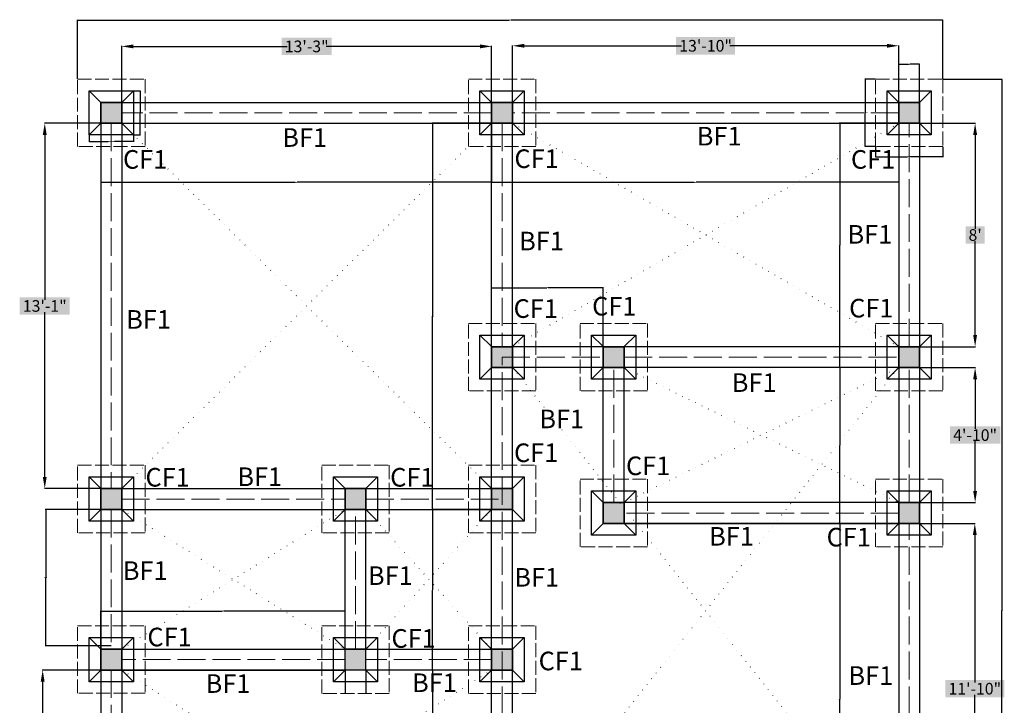
# Model space of a CAD drawing. Units: inches. Extents: x -35 to 832, y -515 to 219.
# Tile 7 of 7: x 409 to 832, y -75 to 219. Entities that reach past the tile are written whole.
import ezdxf

# ---------------------------------------------------------------- set-up
doc = ezdxf.new("R2010")
doc.units = ezdxf.units.IN
doc.header["$MEASUREMENT"] = 0
doc.linetypes.add('ACAD_ISO02W100', pattern=[15, 12, -3])
doc.linetypes.add('ACAD_ISO07W100', pattern=[3, 0, -3])
for name, color, linetype, lineweight in [('S-ANNO-DIMS', 2, 'Continuous', 18), ('S-ANNO-TEXT', 7, 'Continuous', 18), ('S-BEAM', 6, 'Continuous', 25), ('S-BEAM-CNTR', 2, 'ACAD_ISO02W100', 13), ('S-COLS', 4, 'Continuous', 35), ('S-COLS-PATT', 8, 'Continuous', 13), ('S-FNDN', 4, 'Continuous', 25), ('S-FNDN-HIDN', 7, 'ACAD_ISO02W100', 18), ('S-FNDN-REFR', 8, 'ACAD_ISO07W100', 13)]:
    doc.layers.add(name, color=color, linetype=linetype, lineweight=lineweight)
doc.styles.get("Standard").update_dxf_attribs({"font": 'arial.ttf'})
doc.dimstyles.get("Standard").update_dxf_attribs({"dimtxt": 0.18, "dimasz": 0.18, "dimexe": 0.18, "dimexo": 0.0625, "dimgap": 0.09, "dimtad": 0, "dimtih": 1, "dimtoh": 1, "dimdec": 1, "dimzin": 0, "dimdsep": 46, "dimlunit": 4, "dimtxsty": 'Standard', "dimcen": 0.09, "dimclrd": 211, "dimclre": 4, "dimclrt": 3, "dimadec": 0, "dimazin": 0, "dimtfac": 0.5, "dimtdec": 1, "dimtofl": 0, "dimtmove": 0, "dimatfit": 3, "dimfxl": 1, "dimtfill": 2, "dimtfillclr": 61, "dimtolj": 1, "dimtzin": 0, "dimarcsym": 0})

# ---------------------------------------------------------------- blocks, each defined once
blk = doc.blocks.new('*D31')
at = {"layer": 'Defpoints', "color": 0, "transparency": 16777216}
for p in [(786.57, 2.92), (819.29, 2.92), (786.57, -139.08)]:
    blk.add_point(p, dxfattribs=at)
at = {"layer": 'S-ANNO-DIMS', "color": 0, "lineweight": -2, "transparency": 16777216}
for p, q in [((786.63, 2.92), (819.47, 2.92)), ((819.29, -2.08), (819.29, -65.43)), ((819.29, -134.08), (819.29, -70.72)), ((786.63, -139.08), (819.47, -139.08))]:
    blk.add_line(p, q, dxfattribs=at)
at = {"layer": 'S-ANNO-DIMS', "color": 0, "transparency": 16777216}
for points in [[(818.46, -2.08), (820.13, -2.08), (819.29, 2.92)], [(818.46, -134.08), (820.13, -134.08), (819.29, -139.08)]]:
    blk.add_solid(points, dxfattribs=at)
at = {"layer": 'S-ANNO-DIMS', "color": 0, "transparency": 16777216, "insert": (819.29, -68.08), "char_height": 5, "attachment_point": 5, "bg_fill": 1, "box_fill_scale": 1.25, "bg_fill_color": 61, "bg_fill_transparency": 0}
blk.add_mtext('\\A1;11\'-10"', dxfattribs=at)
blk = doc.blocks.new('*D32')
at = {"layer": 'Defpoints', "color": 0, "transparency": 16777216}
for p in [(791.07, 69.92), (819.43, 69.92), (791.07, 11.92)]:
    blk.add_point(p, dxfattribs=at)
at = {"layer": 'S-ANNO-DIMS', "color": 0, "lineweight": -2, "transparency": 16777216}
for p, q in [((791.13, 69.92), (819.61, 69.92)), ((819.43, 64.92), (819.43, 43.57)), ((819.43, 16.92), (819.43, 38.28)), ((791.13, 11.92), (819.61, 11.92))]:
    blk.add_line(p, q, dxfattribs=at)
at = {"layer": 'S-ANNO-DIMS', "color": 0, "transparency": 16777216}
for points in [[(818.6, 64.92), (820.26, 64.92), (819.43, 69.92)], [(818.6, 16.92), (820.26, 16.92), (819.43, 11.92)]]:
    blk.add_solid(points, dxfattribs=at)
at = {"layer": 'S-ANNO-DIMS', "color": 0, "transparency": 16777216, "insert": (819.43, 40.92), "char_height": 5, "attachment_point": 5, "bg_fill": 1, "box_fill_scale": 1.25, "bg_fill_color": 61, "bg_fill_transparency": 0}
blk.add_mtext('\\A1;4\'-10"', dxfattribs=at)
blk = doc.blocks.new('*D33')
at = {"layer": 'Defpoints', "color": 0, "transparency": 16777216}
for p in [(791.07, 174.92), (819.43, 174.92), (791.07, 78.92)]:
    blk.add_point(p, dxfattribs=at)
at = {"layer": 'S-ANNO-DIMS', "color": 0, "lineweight": -2, "transparency": 16777216}
for p, q in [((791.13, 174.92), (819.61, 174.92)), ((819.43, 169.92), (819.43, 129.57)), ((819.43, 83.92), (819.43, 124.28)), ((791.13, 78.92), (819.61, 78.92))]:
    blk.add_line(p, q, dxfattribs=at)
at = {"layer": 'S-ANNO-DIMS', "color": 0, "transparency": 16777216}
for points in [[(818.6, 169.92), (820.27, 169.92), (819.43, 174.92)], [(818.6, 83.92), (820.27, 83.92), (819.43, 78.92)]]:
    blk.add_solid(points, dxfattribs=at)
at = {"layer": 'S-ANNO-DIMS', "color": 0, "transparency": 16777216, "insert": (819.43, 126.92), "char_height": 5, "attachment_point": 5, "bg_fill": 1, "box_fill_scale": 1.25, "bg_fill_color": 61, "bg_fill_transparency": 0}
blk.add_mtext("\\A1;8'", dxfattribs=at)
blk = doc.blocks.new('*D34')
at = {"layer": 'Defpoints', "color": 0, "transparency": 16777216}
for p in [(611.57, 207.98), (452.57, 179.42), (611.57, 179.42)]:
    blk.add_point(p, dxfattribs=at)
at = {"layer": 'S-ANNO-DIMS', "color": 0, "lineweight": -2, "transparency": 16777216}
for p, q in [((452.57, 179.49), (452.57, 208.16)), ((457.57, 207.98), (523.63, 207.98)), ((606.57, 207.98), (540.51, 207.98)), ((611.57, 179.49), (611.57, 208.16))]:
    blk.add_line(p, q, dxfattribs=at)
at = {"layer": 'S-ANNO-DIMS', "color": 0, "transparency": 16777216}
for points in [[(457.57, 208.81), (457.57, 207.14), (452.57, 207.98)], [(606.57, 208.81), (606.57, 207.14), (611.57, 207.98)]]:
    blk.add_solid(points, dxfattribs=at)
at = {"layer": 'S-ANNO-DIMS', "color": 0, "transparency": 16777216, "insert": (532.07, 207.98), "char_height": 5, "attachment_point": 5, "bg_fill": 1, "box_fill_scale": 1.25, "bg_fill_color": 61, "bg_fill_transparency": 0}
blk.add_mtext('\\A1;13\'-3"', dxfattribs=at)
blk = doc.blocks.new('*D35')
at = {"layer": 'Defpoints', "color": 0, "transparency": 16777216}
for p in [(786.57, 208.24), (620.57, 179.42), (786.57, 179.42)]:
    blk.add_point(p, dxfattribs=at)
at = {"layer": 'S-ANNO-DIMS', "color": 0, "lineweight": -2, "transparency": 16777216}
for p, q in [((620.57, 179.49), (620.57, 208.42)), ((625.57, 208.24), (693.19, 208.24)), ((781.57, 208.24), (713.96, 208.24)), ((786.57, 179.49), (786.57, 208.42))]:
    blk.add_line(p, q, dxfattribs=at)
at = {"layer": 'S-ANNO-DIMS', "color": 0, "transparency": 16777216}
for points in [[(625.57, 209.07), (625.57, 207.41), (620.57, 208.24)], [(781.57, 209.07), (781.57, 207.41), (786.57, 208.24)]]:
    blk.add_solid(points, dxfattribs=at)
at = {"layer": 'S-ANNO-DIMS', "color": 0, "transparency": 16777216, "insert": (703.57, 208.24), "char_height": 5, "attachment_point": 5, "bg_fill": 1, "box_fill_scale": 1.25, "bg_fill_color": 61, "bg_fill_transparency": 0}
blk.add_mtext('\\A1;13\'-10"', dxfattribs=at)
blk = doc.blocks.new('*D36')
at = {"layer": 'Defpoints', "color": 0, "transparency": 16777216}
for p in [(448.07, 174.92), (419.47, 17.92), (448.07, 17.92)]:
    blk.add_point(p, dxfattribs=at)
at = {"layer": 'S-ANNO-DIMS', "color": 0, "lineweight": -2, "transparency": 16777216}
for p, q in [((448.01, 174.92), (419.29, 174.92)), ((419.47, 169.92), (419.47, 99.07)), ((419.47, 22.92), (419.47, 93.78)), ((448.01, 17.92), (419.29, 17.92))]:
    blk.add_line(p, q, dxfattribs=at)
at = {"layer": 'S-ANNO-DIMS', "color": 0, "transparency": 16777216}
for points in [[(418.63, 169.92), (420.3, 169.92), (419.47, 174.92)], [(418.63, 22.92), (420.3, 22.92), (419.47, 17.92)]]:
    blk.add_solid(points, dxfattribs=at)
at = {"layer": 'S-ANNO-DIMS', "color": 0, "transparency": 16777216, "insert": (419.47, 96.42), "char_height": 5, "attachment_point": 5, "bg_fill": 1, "box_fill_scale": 1.25, "bg_fill_color": 61, "bg_fill_transparency": 0}
blk.add_mtext('\\A1;13\'-1"', dxfattribs=at)
blk = doc.blocks.new('*D37')
at = {"layer": 'Defpoints', "color": 0, "transparency": 16777216}
for p in [(448.07, 8.92), (419.88, -49.73), (448.07, -49.73)]:
    blk.add_point(p, dxfattribs=at)
at = {"layer": 'S-ANNO-DIMS', "color": 0, "lineweight": -2, "transparency": 16777216}
for p, q in [((448.01, 8.92), (419.7, 8.92)), ((419.88, 8.74), (419.88, -20.21)), ((419.88, -49.55), (419.88, -20.6)), ((448.01, -49.73), (419.7, -49.73))]:
    blk.add_line(p, q, dxfattribs=at)
at = {"layer": 'S-ANNO-DIMS', "color": 0, "transparency": 16777216}
for points in [[(419.85, 8.74), (419.91, 8.74), (419.88, 8.92)], [(419.85, -49.55), (419.91, -49.55), (419.88, -49.73)]]:
    blk.add_solid(points, dxfattribs=at)
at = {"layer": 'S-ANNO-DIMS', "color": 0, "transparency": 16777216, "insert": (419.88, -20.4), "char_height": 0.18, "attachment_point": 5, "bg_fill": 1, "box_fill_scale": 1.25, "bg_fill_color": 61, "bg_fill_transparency": 0}
blk.add_mtext('\\A1;4\'-10{\\H0.5x;\\S1/2;}"', dxfattribs=at)
blk = doc.blocks.new('*D38')
at = {"layer": 'Defpoints', "color": 0, "transparency": 16777216}
for p in [(448.07, -60.08), (418.57, -161.08), (448.07, -161.08)]:
    blk.add_point(p, dxfattribs=at)
at = {"layer": 'S-ANNO-DIMS', "color": 0, "lineweight": -2, "transparency": 16777216}
for p, q in [((448.01, -60.08), (418.39, -60.08)), ((418.57, -65.08), (418.57, -107.93)), ((418.57, -156.08), (418.57, -113.22)), ((448.01, -161.08), (418.39, -161.08))]:
    blk.add_line(p, q, dxfattribs=at)
at = {"layer": 'S-ANNO-DIMS', "color": 0, "transparency": 16777216}
for points in [[(417.74, -65.08), (419.41, -65.08), (418.57, -60.08)], [(417.74, -156.08), (419.41, -156.08), (418.57, -161.08)]]:
    blk.add_solid(points, dxfattribs=at)
at = {"layer": 'S-ANNO-DIMS', "color": 0, "transparency": 16777216, "insert": (418.57, -110.58), "char_height": 5, "attachment_point": 5, "bg_fill": 1, "box_fill_scale": 1.25, "bg_fill_color": 61, "bg_fill_transparency": 0}
blk.add_mtext('\\A1;8\'-5"', dxfattribs=at)
blk = doc.blocks.new('CF1-TAPERED-FOOTING')
for p, q in [((0, 19), (19, 19)), ((0, 0), (0, 19)), ((0, 19), (5, 14)), ((14, 14), (19, 19)), ((19, 19), (19, 0)), ((0, 0), (5, 5)), ((14, 5), (19, 0)), ((19, 0), (0, 0))]:
    blk.add_line(p, q)
blk = doc.blocks.new('CF1-FOOTING-LIMIT')
at = {"ltscale": 0.5}
for p, q in [((0, 29), (29, 29)), ((0, 0), (0, 29)), ((29, 29), (29, 0)), ((29, 0), (0, 0))]:
    blk.add_line(p, q, dxfattribs=at)
blk = doc.blocks.new('*D57')
at = {"layer": 'Defpoints', "color": 0, "transparency": 16777216}
for p in [(438.57, 169.92), (457.57, 169.92), (457.57, 167.07)]:
    blk.add_point(p, dxfattribs=at)
at = {"layer": 'S-ANNO-DIMS', "color": 4, "lineweight": -2, "transparency": 16777216}
for p, q in [((438.57, 169.86), (438.57, 166.89)), ((457.57, 169.86), (457.57, 166.89))]:
    blk.add_line(p, q, dxfattribs=at)
at = {"layer": 'S-ANNO-DIMS', "color": 211, "lineweight": -2, "transparency": 16777216}
for p, q in [((438.75, 167.07), (446.71, 167.07)), ((457.39, 167.07), (449.44, 167.07))]:
    blk.add_line(p, q, dxfattribs=at)
at = {"layer": 'S-ANNO-DIMS', "color": 211, "transparency": 16777216}
for points in [[(438.75, 167.1), (438.75, 167.04), (438.57, 167.07)], [(457.39, 167.1), (457.39, 167.04), (457.57, 167.07)]]:
    blk.add_solid(points, dxfattribs=at)
at = {"layer": 'S-ANNO-DIMS', "color": 3, "transparency": 16777216, "insert": (448.07, 167.07), "char_height": 0.18, "attachment_point": 5, "bg_fill": 1, "box_fill_scale": 1.25, "bg_fill_color": 61, "bg_fill_transparency": 0}
blk.add_mtext('\\A1;CF1 TAPER 1\'-7" TYP.', dxfattribs=at)
blk = doc.blocks.new('*D58')
at = {"layer": 'Defpoints', "color": 0, "transparency": 16777216}
for p in [(457.57, 188.92), (460.42, 188.92), (457.57, 169.92)]:
    blk.add_point(p, dxfattribs=at)
at = {"layer": 'S-ANNO-DIMS', "color": 4, "lineweight": -2, "transparency": 16777216}
for p, q in [((457.63, 188.92), (460.6, 188.92)), ((457.63, 169.92), (460.6, 169.92))]:
    blk.add_line(p, q, dxfattribs=at)
at = {"layer": 'S-ANNO-DIMS', "color": 211, "lineweight": -2, "transparency": 16777216}
for p, q in [((460.42, 188.74), (460.42, 179.61)), ((460.42, 170.1), (460.42, 179.24))]:
    blk.add_line(p, q, dxfattribs=at)
at = {"layer": 'S-ANNO-DIMS', "color": 211, "transparency": 16777216}
for points in [[(460.39, 188.74), (460.45, 188.74), (460.42, 188.92)], [(460.39, 170.1), (460.45, 170.1), (460.42, 169.92)]]:
    blk.add_solid(points, dxfattribs=at)
at = {"layer": 'S-ANNO-DIMS', "color": 3, "transparency": 16777216, "insert": (460.42, 179.42), "char_height": 0.18, "attachment_point": 5, "bg_fill": 1, "box_fill_scale": 1.25, "bg_fill_color": 61, "bg_fill_transparency": 0}
blk.add_mtext('\\A1;1\'-7" TYP.', dxfattribs=at)
blk = doc.blocks.new('*D59')
at = {"layer": 'Defpoints', "color": 0, "transparency": 16777216}
for p in [(772.22, 193.92), (776.57, 193.92), (776.57, 164.92)]:
    blk.add_point(p, dxfattribs=at)
at = {"layer": 'S-ANNO-DIMS', "color": 4, "lineweight": -2, "transparency": 16777216}
for p, q in [((776.51, 193.92), (772.04, 193.92)), ((776.51, 164.92), (772.04, 164.92))]:
    blk.add_line(p, q, dxfattribs=at)
at = {"layer": 'S-ANNO-DIMS', "color": 211, "lineweight": -2, "transparency": 16777216}
for p, q in [((772.22, 193.74), (772.22, 179.61)), ((772.22, 165.1), (772.22, 179.24))]:
    blk.add_line(p, q, dxfattribs=at)
at = {"layer": 'S-ANNO-DIMS', "color": 211, "transparency": 16777216}
for points in [[(772.19, 193.74), (772.25, 193.74), (772.22, 193.92)], [(772.19, 165.1), (772.25, 165.1), (772.22, 164.92)]]:
    blk.add_solid(points, dxfattribs=at)
at = {"layer": 'S-ANNO-DIMS', "color": 3, "transparency": 16777216, "insert": (772.22, 179.42), "char_height": 0.18, "attachment_point": 5, "bg_fill": 1, "box_fill_scale": 1.25, "bg_fill_color": 61, "bg_fill_transparency": 0}
blk.add_mtext('\\A1;CF1 LIMIT 2\'-5" TYP.', dxfattribs=at)
blk = doc.blocks.new('*D60')
at = {"layer": 'Defpoints', "color": 0, "transparency": 16777216}
for p in [(776.57, 164.92), (805.57, 164.92), (776.57, 160.57)]:
    blk.add_point(p, dxfattribs=at)
at = {"layer": 'S-ANNO-DIMS', "color": 4, "lineweight": -2, "transparency": 16777216}
for p, q in [((776.57, 164.86), (776.57, 160.39)), ((805.57, 164.86), (805.57, 160.39))]:
    blk.add_line(p, q, dxfattribs=at)
at = {"layer": 'S-ANNO-DIMS', "color": 211, "lineweight": -2, "transparency": 16777216}
for p, q in [((776.75, 160.57), (790.43, 160.57)), ((805.39, 160.57), (791.71, 160.57))]:
    blk.add_line(p, q, dxfattribs=at)
at = {"layer": 'S-ANNO-DIMS', "color": 211, "transparency": 16777216}
for points in [[(776.75, 160.6), (776.75, 160.54), (776.57, 160.57)], [(805.39, 160.6), (805.39, 160.54), (805.57, 160.57)]]:
    blk.add_solid(points, dxfattribs=at)
at = {"layer": 'S-ANNO-DIMS', "color": 3, "transparency": 16777216, "insert": (791.07, 160.57), "char_height": 0.18, "attachment_point": 5, "bg_fill": 1, "box_fill_scale": 1.25, "bg_fill_color": 61, "bg_fill_transparency": 0}
blk.add_mtext('\\A1;2\'-5" TYP.', dxfattribs=at)
blk = doc.blocks.new('*D136')
at = {"layer": 'Defpoints', "color": 0, "transparency": 16777216}
for p in [(548.57, -34.73), (443.57, -60.08), (548.57, -60.08)]:
    blk.add_point(p, dxfattribs=at)
at = {"layer": 'S-ANNO-DIMS', "color": 4, "lineweight": -2, "transparency": 16777216}
for p, q in [((443.57, -60.01), (443.57, -34.55)), ((548.57, -60.01), (548.57, -34.55))]:
    blk.add_line(p, q, dxfattribs=at)
at = {"layer": 'S-ANNO-DIMS', "color": 211, "lineweight": -2, "transparency": 16777216}
for p, q in [((443.75, -34.73), (495.74, -34.73)), ((548.39, -34.73), (496.4, -34.73))]:
    blk.add_line(p, q, dxfattribs=at)
at = {"layer": 'S-ANNO-DIMS', "color": 211, "transparency": 16777216}
for points in [[(443.75, -34.7), (443.75, -34.76), (443.57, -34.73)], [(548.39, -34.7), (548.39, -34.76), (548.57, -34.73)]]:
    blk.add_solid(points, dxfattribs=at)
at = {"layer": 'S-ANNO-DIMS', "color": 3, "transparency": 16777216, "insert": (496.07, -34.73), "char_height": 0.18, "attachment_point": 5, "bg_fill": 1, "box_fill_scale": 1.25, "bg_fill_color": 61, "bg_fill_transparency": 0}
blk.add_mtext('\\A1;8\'-9"', dxfattribs=at)
blk = doc.blocks.new('*D137')
at = {"layer": 'Defpoints', "color": 0, "transparency": 16777216}
for p in [(659.57, 104.27), (611.57, 78.92), (659.57, 78.92)]:
    blk.add_point(p, dxfattribs=at)
at = {"layer": 'S-ANNO-DIMS', "color": 4, "lineweight": -2, "transparency": 16777216}
for p, q in [((611.57, 78.99), (611.57, 104.45)), ((659.57, 78.99), (659.57, 104.45))]:
    blk.add_line(p, q, dxfattribs=at)
at = {"layer": 'S-ANNO-DIMS', "color": 211, "lineweight": -2, "transparency": 16777216}
for p, q in [((611.75, 104.27), (635.24, 104.27)), ((659.39, 104.27), (635.9, 104.27))]:
    blk.add_line(p, q, dxfattribs=at)
at = {"layer": 'S-ANNO-DIMS', "color": 211, "transparency": 16777216}
for points in [[(611.75, 104.3), (611.75, 104.24), (611.57, 104.27)], [(659.39, 104.3), (659.39, 104.24), (659.57, 104.27)]]:
    blk.add_solid(points, dxfattribs=at)
at = {"layer": 'S-ANNO-DIMS', "color": 3, "transparency": 16777216, "insert": (635.57, 104.27), "char_height": 0.18, "attachment_point": 5, "bg_fill": 1, "box_fill_scale": 1.25, "bg_fill_color": 61, "bg_fill_transparency": 0}
blk.add_mtext('\\A1;4\'-0"', dxfattribs=at)
blk = doc.blocks.new('*D138')
at = {"layer": 'Defpoints', "color": 0, "transparency": 16777216}
for p in [(795.57, 200.27), (786.57, 174.92), (795.57, 174.92)]:
    blk.add_point(p, dxfattribs=at)
at = {"layer": 'S-ANNO-DIMS', "color": 4, "lineweight": -2, "transparency": 16777216}
for p, q in [((786.57, 174.99), (786.57, 200.45)), ((795.57, 174.99), (795.57, 200.45))]:
    blk.add_line(p, q, dxfattribs=at)
at = {"layer": 'S-ANNO-DIMS', "color": 211, "lineweight": -2, "transparency": 16777216}
for p, q in [((786.75, 200.27), (790.74, 200.27)), ((795.39, 200.27), (791.4, 200.27))]:
    blk.add_line(p, q, dxfattribs=at)
at = {"layer": 'S-ANNO-DIMS', "color": 211, "transparency": 16777216}
for points in [[(786.75, 200.3), (786.75, 200.24), (786.57, 200.27)], [(795.39, 200.3), (795.39, 200.24), (795.57, 200.27)]]:
    blk.add_solid(points, dxfattribs=at)
at = {"layer": 'S-ANNO-DIMS', "color": 3, "transparency": 16777216, "insert": (791.07, 200.27), "char_height": 0.18, "attachment_point": 5, "bg_fill": 1, "box_fill_scale": 1.25, "bg_fill_color": 61, "bg_fill_transparency": 0}
blk.add_mtext('\\A1;0\'-9"', dxfattribs=at)
blk = doc.blocks.new('*D139')
at = {"layer": 'Defpoints', "color": 0, "transparency": 16777216}
for p in [(805.57, 219.27), (433.57, 193.92), (805.57, 193.92)]:
    blk.add_point(p, dxfattribs=at)
at = {"layer": 'S-ANNO-DIMS', "color": 4, "lineweight": -2, "transparency": 16777216}
for p, q in [((433.57, 193.99), (433.57, 219.45)), ((805.57, 193.99), (805.57, 219.45))]:
    blk.add_line(p, q, dxfattribs=at)
at = {"layer": 'S-ANNO-DIMS', "color": 211, "lineweight": -2, "transparency": 16777216}
for p, q in [((433.75, 219.27), (619.17, 219.27)), ((805.39, 219.27), (619.97, 219.27))]:
    blk.add_line(p, q, dxfattribs=at)
at = {"layer": 'S-ANNO-DIMS', "color": 211, "transparency": 16777216}
for points in [[(433.75, 219.3), (433.75, 219.24), (433.57, 219.27)], [(805.39, 219.3), (805.39, 219.24), (805.57, 219.27)]]:
    blk.add_solid(points, dxfattribs=at)
at = {"layer": 'S-ANNO-DIMS', "color": 3, "transparency": 16777216, "insert": (619.57, 219.27), "char_height": 0.18, "attachment_point": 5, "bg_fill": 1, "box_fill_scale": 1.25, "bg_fill_color": 61, "bg_fill_transparency": 0}
blk.add_mtext('\\A1;31\'-0"', dxfattribs=at)
blk = doc.blocks.new('*D140')
at = {"layer": 'Defpoints', "color": 0, "transparency": 16777216}
for p in [(805.57, 193.92), (805.57, -263.08), (830.92, -263.08)]:
    blk.add_point(p, dxfattribs=at)
at = {"layer": 'S-ANNO-DIMS', "color": 4, "lineweight": -2, "transparency": 16777216}
for p, q in [((805.63, 193.92), (831.1, 193.92)), ((805.63, -263.08), (831.1, -263.08))]:
    blk.add_line(p, q, dxfattribs=at)
at = {"layer": 'S-ANNO-DIMS', "color": 211, "lineweight": -2, "transparency": 16777216}
for p, q in [((830.92, 193.74), (830.92, -34.39)), ((830.92, -262.9), (830.92, -34.76))]:
    blk.add_line(p, q, dxfattribs=at)
at = {"layer": 'S-ANNO-DIMS', "color": 211, "transparency": 16777216}
for points in [[(830.89, 193.74), (830.95, 193.74), (830.92, 193.92)], [(830.89, -262.9), (830.95, -262.9), (830.92, -263.08)]]:
    blk.add_solid(points, dxfattribs=at)
at = {"layer": 'S-ANNO-DIMS', "color": 3, "transparency": 16777216, "insert": (830.92, -34.58), "char_height": 0.18, "attachment_point": 5, "bg_fill": 1, "box_fill_scale": 1.25, "bg_fill_color": 61, "bg_fill_transparency": 0}
blk.add_mtext('\\A1;38\'-1"', dxfattribs=at)
blk = doc.blocks.new('*D141')
at = {"layer": 'Defpoints', "color": 0, "transparency": 16777216}
for p in [(443.57, 174.92), (611.57, 174.92), (443.57, 149.57)]:
    blk.add_point(p, dxfattribs=at)
at = {"layer": 'S-ANNO-DIMS', "color": 4, "lineweight": -2, "transparency": 16777216}
for p, q in [((443.57, 174.86), (443.57, 149.39)), ((611.57, 174.86), (611.57, 149.39))]:
    blk.add_line(p, q, dxfattribs=at)
at = {"layer": 'S-ANNO-DIMS', "color": 211, "lineweight": -2, "transparency": 16777216}
for p, q in [((443.75, 149.57), (527.18, 149.57)), ((611.39, 149.57), (527.96, 149.57))]:
    blk.add_line(p, q, dxfattribs=at)
at = {"layer": 'S-ANNO-DIMS', "color": 211, "transparency": 16777216}
for points in [[(443.75, 149.6), (443.75, 149.54), (443.57, 149.57)], [(611.39, 149.6), (611.39, 149.54), (611.57, 149.57)]]:
    blk.add_solid(points, dxfattribs=at)
at = {"layer": 'S-ANNO-DIMS', "color": 3, "transparency": 16777216, "insert": (527.57, 149.57), "char_height": 0.18, "attachment_point": 5, "bg_fill": 1, "box_fill_scale": 1.25, "bg_fill_color": 61, "bg_fill_transparency": 0}
blk.add_mtext('\\A1;14\'-0"', dxfattribs=at)
blk = doc.blocks.new('*D142')
at = {"layer": 'Defpoints', "color": 0, "transparency": 16777216}
for p in [(611.57, 174.92), (786.57, 174.92), (611.57, 149.57)]:
    blk.add_point(p, dxfattribs=at)
at = {"layer": 'S-ANNO-DIMS', "color": 4, "lineweight": -2, "transparency": 16777216}
for p, q in [((611.57, 174.86), (611.57, 149.39)), ((786.57, 174.86), (786.57, 149.39))]:
    blk.add_line(p, q, dxfattribs=at)
at = {"layer": 'S-ANNO-DIMS', "color": 211, "lineweight": -2, "transparency": 16777216}
for p, q in [((611.75, 149.57), (698.68, 149.57)), ((786.39, 149.57), (699.46, 149.57))]:
    blk.add_line(p, q, dxfattribs=at)
at = {"layer": 'S-ANNO-DIMS', "color": 211, "transparency": 16777216}
for points in [[(611.75, 149.6), (611.75, 149.54), (611.57, 149.57)], [(786.39, 149.6), (786.39, 149.54), (786.57, 149.57)]]:
    blk.add_solid(points, dxfattribs=at)
at = {"layer": 'S-ANNO-DIMS', "color": 3, "transparency": 16777216, "insert": (699.07, 149.57), "char_height": 0.18, "attachment_point": 5, "bg_fill": 1, "box_fill_scale": 1.25, "bg_fill_color": 61, "bg_fill_transparency": 0}
blk.add_mtext('\\A1;14\'-7"', dxfattribs=at)
blk = doc.blocks.new('*D143')
at = {"layer": 'Defpoints', "color": 0, "transparency": 16777216}
for p in [(586.22, 174.92), (611.57, 174.92), (611.57, 8.92)]:
    blk.add_point(p, dxfattribs=at)
at = {"layer": 'S-ANNO-DIMS', "color": 4, "lineweight": -2, "transparency": 16777216}
for p, q in [((611.51, 174.92), (586.04, 174.92)), ((611.51, 8.92), (586.04, 8.92))]:
    blk.add_line(p, q, dxfattribs=at)
at = {"layer": 'S-ANNO-DIMS', "color": 211, "lineweight": -2, "transparency": 16777216}
for p, q in [((586.22, 174.74), (586.22, 92.11)), ((586.22, 9.1), (586.22, 91.74))]:
    blk.add_line(p, q, dxfattribs=at)
at = {"layer": 'S-ANNO-DIMS', "color": 211, "transparency": 16777216}
for points in [[(586.19, 174.74), (586.25, 174.74), (586.22, 174.92)], [(586.19, 9.1), (586.25, 9.1), (586.22, 8.92)]]:
    blk.add_solid(points, dxfattribs=at)
at = {"layer": 'S-ANNO-DIMS', "color": 3, "transparency": 16777216, "insert": (586.22, 91.92), "char_height": 0.18, "attachment_point": 5, "bg_fill": 1, "box_fill_scale": 1.25, "bg_fill_color": 61, "bg_fill_transparency": 0}
blk.add_mtext('\\A1;13\'-10"', dxfattribs=at)
blk = doc.blocks.new('*D144')
at = {"layer": 'Defpoints', "color": 0, "transparency": 16777216}
for p in [(586.22, 8.92), (611.57, 8.92), (611.57, -60.08)]:
    blk.add_point(p, dxfattribs=at)
at = {"layer": 'S-ANNO-DIMS', "color": 4, "lineweight": -2, "transparency": 16777216}
for p, q in [((611.51, 8.92), (586.04, 8.92)), ((611.51, -60.08), (586.04, -60.08))]:
    blk.add_line(p, q, dxfattribs=at)
at = {"layer": 'S-ANNO-DIMS', "color": 211, "lineweight": -2, "transparency": 16777216}
for p, q in [((586.22, 8.74), (586.22, -25.39)), ((586.22, -59.9), (586.22, -25.76))]:
    blk.add_line(p, q, dxfattribs=at)
at = {"layer": 'S-ANNO-DIMS', "color": 211, "transparency": 16777216}
for points in [[(586.19, 8.74), (586.25, 8.74), (586.22, 8.92)], [(586.19, -59.9), (586.25, -59.9), (586.22, -60.08)]]:
    blk.add_solid(points, dxfattribs=at)
at = {"layer": 'S-ANNO-DIMS', "color": 3, "transparency": 16777216, "insert": (586.22, -25.58), "char_height": 0.18, "attachment_point": 5, "bg_fill": 1, "box_fill_scale": 1.25, "bg_fill_color": 61, "bg_fill_transparency": 0}
blk.add_mtext('\\A1;5\'-9"', dxfattribs=at)
blk = doc.blocks.new('*D145')
at = {"layer": 'Defpoints', "color": 0, "transparency": 16777216}
for p in [(586.22, -60.08), (611.57, -60.08), (611.57, -170.08)]:
    blk.add_point(p, dxfattribs=at)
at = {"layer": 'S-ANNO-DIMS', "color": 4, "lineweight": -2, "transparency": 16777216}
for p, q in [((611.51, -60.08), (586.04, -60.08)), ((611.51, -170.08), (586.04, -170.08))]:
    blk.add_line(p, q, dxfattribs=at)
at = {"layer": 'S-ANNO-DIMS', "color": 211, "lineweight": -2, "transparency": 16777216}
for p, q in [((586.22, -60.26), (586.22, -114.89)), ((586.22, -169.9), (586.22, -115.26))]:
    blk.add_line(p, q, dxfattribs=at)
at = {"layer": 'S-ANNO-DIMS', "color": 211, "transparency": 16777216}
for points in [[(586.19, -60.26), (586.25, -60.26), (586.22, -60.08)], [(586.19, -169.9), (586.25, -169.9), (586.22, -170.08)]]:
    blk.add_solid(points, dxfattribs=at)
at = {"layer": 'S-ANNO-DIMS', "color": 3, "transparency": 16777216, "insert": (586.22, -115.08), "char_height": 0.18, "attachment_point": 5, "bg_fill": 1, "box_fill_scale": 1.25, "bg_fill_color": 61, "bg_fill_transparency": 0}
blk.add_mtext('\\A1;9\'-2"', dxfattribs=at)
blk = doc.blocks.new('*D146')
at = {"layer": 'Defpoints', "color": 0, "transparency": 16777216}
for p in [(761.22, 174.92), (786.57, 174.92), (786.57, 69.92)]:
    blk.add_point(p, dxfattribs=at)
at = {"layer": 'S-ANNO-DIMS', "color": 4, "lineweight": -2, "transparency": 16777216}
for p, q in [((786.51, 174.92), (761.04, 174.92)), ((786.51, 69.92), (761.04, 69.92))]:
    blk.add_line(p, q, dxfattribs=at)
at = {"layer": 'S-ANNO-DIMS', "color": 211, "lineweight": -2, "transparency": 16777216}
for p, q in [((761.22, 174.74), (761.22, 122.61)), ((761.22, 70.1), (761.22, 122.24))]:
    blk.add_line(p, q, dxfattribs=at)
at = {"layer": 'S-ANNO-DIMS', "color": 211, "transparency": 16777216}
for points in [[(761.19, 174.74), (761.25, 174.74), (761.22, 174.92)], [(761.19, 70.1), (761.25, 70.1), (761.22, 69.92)]]:
    blk.add_solid(points, dxfattribs=at)
at = {"layer": 'S-ANNO-DIMS', "color": 3, "transparency": 16777216, "insert": (761.22, 122.42), "char_height": 0.18, "attachment_point": 5, "bg_fill": 1, "box_fill_scale": 1.25, "bg_fill_color": 61, "bg_fill_transparency": 0}
blk.add_mtext('\\A1;8\'-9"', dxfattribs=at)
blk = doc.blocks.new('*D147')
at = {"layer": 'Defpoints', "color": 0, "transparency": 16777216}
for p in [(761.22, 69.92), (786.57, 69.92), (786.57, 2.92)]:
    blk.add_point(p, dxfattribs=at)
at = {"layer": 'S-ANNO-DIMS', "color": 4, "lineweight": -2, "transparency": 16777216}
for p, q in [((786.51, 69.92), (761.04, 69.92)), ((786.51, 2.92), (761.04, 2.92))]:
    blk.add_line(p, q, dxfattribs=at)
at = {"layer": 'S-ANNO-DIMS', "color": 211, "lineweight": -2, "transparency": 16777216}
for p, q in [((761.22, 69.74), (761.22, 36.61)), ((761.22, 3.1), (761.22, 36.24))]:
    blk.add_line(p, q, dxfattribs=at)
at = {"layer": 'S-ANNO-DIMS', "color": 211, "transparency": 16777216}
for points in [[(761.19, 69.74), (761.25, 69.74), (761.22, 69.92)], [(761.19, 3.1), (761.25, 3.1), (761.22, 2.92)]]:
    blk.add_solid(points, dxfattribs=at)
at = {"layer": 'S-ANNO-DIMS', "color": 3, "transparency": 16777216, "insert": (761.22, 36.42), "char_height": 0.18, "attachment_point": 5, "bg_fill": 1, "box_fill_scale": 1.25, "bg_fill_color": 61, "bg_fill_transparency": 0}
blk.add_mtext('\\A1;5\'-7"', dxfattribs=at)
blk = doc.blocks.new('*D148')
at = {"layer": 'Defpoints', "color": 0, "transparency": 16777216}
for p in [(761.22, 2.92), (786.57, 2.92), (786.57, -148.08)]:
    blk.add_point(p, dxfattribs=at)
at = {"layer": 'S-ANNO-DIMS', "color": 4, "lineweight": -2, "transparency": 16777216}
for p, q in [((786.51, 2.92), (761.04, 2.92)), ((786.51, -148.08), (761.04, -148.08))]:
    blk.add_line(p, q, dxfattribs=at)
at = {"layer": 'S-ANNO-DIMS', "color": 211, "lineweight": -2, "transparency": 16777216}
for p, q in [((761.22, 2.74), (761.22, -72.39)), ((761.22, -147.9), (761.22, -72.76))]:
    blk.add_line(p, q, dxfattribs=at)
at = {"layer": 'S-ANNO-DIMS', "color": 211, "transparency": 16777216}
for points in [[(761.19, 2.74), (761.25, 2.74), (761.22, 2.92)], [(761.19, -147.9), (761.25, -147.9), (761.22, -148.08)]]:
    blk.add_solid(points, dxfattribs=at)
at = {"layer": 'S-ANNO-DIMS', "color": 3, "transparency": 16777216, "insert": (761.22, -72.58), "char_height": 0.18, "attachment_point": 5, "bg_fill": 1, "box_fill_scale": 1.25, "bg_fill_color": 61, "bg_fill_transparency": 0}
blk.add_mtext('\\A1;12\'-7"', dxfattribs=at)

msp = doc.modelspace()

# ---------------------------------------------------------------- hatches: boundary and pattern name
at = {"layer": 'S-COLS-PATT'}
h = msp.add_hatch(color=256, dxfattribs=at)
h.dxf.hatch_style = 1
h.paths.add_polyline_path([(443.57, 183.92), (443.57, 174.92), (452.57, 174.92), (452.57, 183.92)])
h.paths.add_polyline_path([(620.57, 183.92), (611.57, 183.92), (611.57, 174.92), (620.57, 174.92)])
h.paths.add_polyline_path([(786.57, 183.92), (786.57, 174.92), (795.57, 174.92), (795.57, 183.92)])
h.paths.add_polyline_path([(620.57, 78.92), (611.57, 78.92), (611.57, 69.92), (620.57, 69.92)])
h.paths.add_polyline_path([(659.57, 78.92), (659.57, 69.92), (668.57, 69.92), (668.57, 78.92)])
h.paths.add_polyline_path([(795.57, 78.92), (786.57, 78.92), (786.57, 69.92), (795.57, 69.92)])
h.paths.add_polyline_path([(668.57, 11.92), (659.57, 11.92), (659.57, 2.92), (668.57, 2.92)])
h.paths.add_polyline_path([(795.57, 11.92), (786.57, 11.92), (786.57, 2.92), (795.57, 2.92)])
h.paths.add_polyline_path([(611.57, 17.92), (611.57, 8.92), (620.57, 8.92), (620.57, 17.92)])
h.paths.add_polyline_path([(557.57, 17.92), (548.57, 17.92), (548.57, 8.92), (557.57, 8.92)])
h.paths.add_polyline_path([(443.57, 8.92), (452.57, 8.92), (452.57, 17.92), (443.57, 17.92)])
h.paths.add_polyline_path([(443.57, -51.08), (443.57, -60.08), (452.57, -60.08), (452.57, -51.08)])
h.paths.add_polyline_path([(557.57, -51.08), (548.57, -51.08), (548.57, -60.08), (557.57, -60.08)])
h.paths.add_polyline_path([(620.57, -60.08), (620.57, -51.08), (611.57, -51.08), (611.57, -60.08)])
h.paths.add_polyline_path([(620.57, -139.08), (611.57, -139.08), (611.57, -148.08), (620.57, -148.08)])
h.paths.add_polyline_path([(786.57, -148.08), (795.57, -148.08), (795.57, -139.08), (786.57, -139.08)])
h.paths.add_polyline_path([(443.57, -161.08), (443.57, -170.08), (452.57, -170.08), (452.57, -161.08)])
h.paths.add_polyline_path([(611.57, -161.08), (611.57, -170.08), (620.57, -170.08), (620.57, -161.08)])
h.paths.add_polyline_path([(620.57, -244.08), (611.57, -244.08), (611.57, -253.08), (620.57, -253.08)])
h.paths.add_polyline_path([(786.57, -244.08), (786.57, -253.08), (795.57, -253.08), (795.57, -244.08)])

# ---------------------------------------------------------------- linework, layer by layer
at = {"layer": 'S-BEAM'}
for p, q in [((443.57, 183.92), (620.57, 183.92)), ((443.57, 183.92), (443.57, 8.92)), ((620.57, 183.92), (795.57, 183.92)), ((795.57, 183.92), (795.57, 78.92)), ((452.57, 174.92), (611.57, 174.92)), ((452.57, 174.92), (452.57, 17.92)), ((611.57, 69.92), (611.57, 174.92)), ((620.57, 78.92), (620.57, 174.92)), ((620.57, 174.92), (786.57, 174.92)), ((786.57, 174.92), (786.57, 78.92)), ((611.57, -142.58), (611.57, 78.92)), ((786.57, 78.92), (611.57, 78.92)), ((795.57, 78.92), (795.57, 11.92)), ((620.57, -142.58), (620.57, 69.92)), ((659.57, 69.92), (620.57, 69.92)), ((659.57, 2.92), (659.57, 69.92)), ((786.57, 69.92), (668.57, 69.92)), ((668.57, 11.92), (668.57, 69.92)), ((786.57, 69.92), (786.57, 11.92)), ((452.57, 17.92), (620.57, 17.92)), ((443.57, 8.92), (443.57, -51.08)), ((452.57, 8.92), (548.57, 8.92)), ((452.57, 8.92), (452.57, -51.08)), ((548.57, -60.08), (548.57, 8.92)), ((557.57, 8.92), (611.57, 8.92)), ((557.57, -60.08), (557.57, 8.92)), ((786.57, 11.92), (668.57, 11.92)), ((795.57, 11.92), (795.57, -139.08)), ((659.57, 2.92), (786.57, 2.92)), ((786.57, 2.92), (668.57, 2.92)), ((786.57, 2.92), (786.57, -139.08)), ((443.57, -51.08), (443.57, -170.08)), ((452.57, -51.08), (548.57, -51.08)), ((557.57, -51.08), (620.57, -51.08)), ((452.57, -60.08), (548.57, -60.08)), ((452.57, -60.08), (452.57, -161.08)), ((611.57, -60.08), (452.57, -60.08)), ((795.57, -60.08), (795.57, -253.08))]:
    msp.add_line(p, q, dxfattribs=at)
at = {"layer": 'S-BEAM-CNTR'}
for p, q in [((611.57, 179.42), (452.57, 179.42)), ((786.57, 179.42), (620.57, 179.42)), ((448.07, 174.92), (448.07, 17.92)), ((616.07, 174.92), (616.07, 78.92)), ((791.07, 78.92), (791.07, 174.92)), ((616.07, 74.42), (659.57, 74.42)), ((616.07, -139.08), (616.07, 74.42)), ((668.57, 74.42), (786.57, 74.42)), ((664.07, 11.92), (664.07, 69.92)), ((791.07, 11.92), (791.07, 69.92)), ((452.57, 13.42), (548.57, 13.42)), ((557.57, 13.42), (616.07, 13.42)), ((448.07, 8.92), (448.07, -51.08)), ((553.07, -51.08), (553.07, 8.92)), ((786.57, 7.42), (668.57, 7.42)), ((791.07, -139.08), (791.07, 2.92)), ((548.57, -55.58), (452.57, -55.58)), ((611.57, -55.58), (557.57, -55.58)), ((448.07, -60.08), (448.07, -161.08))]:
    msp.add_line(p, q, dxfattribs=at)
at = {"layer": 'S-COLS'}
for p, q in [((443.57, 183.92), (452.57, 183.92)), ((443.57, 174.92), (443.57, 183.92)), ((452.57, 183.92), (452.57, 174.92)), ((611.57, 183.92), (620.57, 183.92)), ((611.57, 174.92), (611.57, 183.92)), ((620.57, 183.92), (620.57, 174.92)), ((786.57, 183.92), (795.57, 183.92)), ((786.57, 174.92), (786.57, 183.92)), ((795.57, 183.92), (795.57, 174.92)), ((452.57, 174.92), (443.57, 174.92)), ((620.57, 174.92), (611.57, 174.92)), ((795.57, 174.92), (786.57, 174.92)), ((611.57, 78.92), (620.57, 78.92)), ((611.57, 69.92), (611.57, 78.92)), ((620.57, 78.92), (620.57, 69.92)), ((659.57, 78.92), (668.57, 78.92)), ((659.57, 69.92), (659.57, 78.92)), ((668.57, 78.92), (668.57, 69.92)), ((786.57, 78.92), (795.57, 78.92)), ((786.57, 69.92), (786.57, 78.92)), ((795.57, 78.92), (795.57, 69.92)), ((620.57, 69.92), (611.57, 69.92)), ((668.57, 69.92), (659.57, 69.92)), ((795.57, 69.92), (786.57, 69.92)), ((443.57, 17.92), (452.57, 17.92)), ((443.57, 8.92), (443.57, 17.92)), ((452.57, 17.92), (452.57, 8.92)), ((548.57, 17.92), (557.57, 17.92)), ((548.57, 8.92), (548.57, 17.92)), ((557.57, 17.92), (557.57, 8.92)), ((620.57, 17.92), (611.57, 17.92)), ((611.57, 17.92), (620.57, 17.92)), ((611.57, 8.92), (611.57, 17.92)), ((620.57, 8.92), (620.57, 17.92)), ((620.57, 17.92), (620.57, 8.92)), ((452.57, 8.92), (443.57, 8.92)), ((557.57, 8.92), (548.57, 8.92)), ((620.57, 8.92), (611.57, 8.92)), ((659.57, 11.92), (668.57, 11.92)), ((659.57, 2.92), (659.57, 11.92)), ((668.57, 11.92), (668.57, 2.92)), ((786.57, 11.92), (795.57, 11.92)), ((786.57, 2.92), (786.57, 11.92)), ((786.57, 11.92), (795.57, 11.92)), ((795.57, 11.92), (795.57, 2.92)), ((668.57, 2.92), (659.57, 2.92)), ((795.57, 2.92), (786.57, 2.92)), ((443.57, -51.08), (452.57, -51.08)), ((443.57, -60.08), (443.57, -51.08)), ((452.57, -51.08), (452.57, -60.08)), ((548.57, -51.08), (557.57, -51.08)), ((620.57, -51.08), (611.57, -51.08)), ((611.57, -51.08), (620.57, -51.08)), ((611.57, -60.08), (611.57, -51.08)), ((620.57, -60.08), (620.57, -51.08)), ((620.57, -51.08), (620.57, -60.08)), ((452.57, -60.08), (443.57, -60.08)), ((620.57, -60.08), (611.57, -60.08))]:
    msp.add_line(p, q, dxfattribs=at)
at = {"layer": 'S-FNDN'}
for p, q in [((548.57, -60.08), (548.57, -70.08)), ((557.57, -60.08), (557.57, -70.08))]:
    msp.add_line(p, q, dxfattribs=at)
at = {"layer": 'S-FNDN-REFR'}
for p, q in [((452.57, 174.92), (611.57, 17.92)), ((452.57, 17.92), (611.57, 174.92)), ((620.57, 174.92), (786.57, 78.92)), ((620.57, 78.92), (786.57, 174.92)), ((620.57, 69.92), (786.57, -139.08)), ((620.57, -139.08), (786.57, 69.92)), ((668.57, 69.92), (786.57, 11.92)), ((668.57, 11.92), (786.57, 69.92)), ((452.57, 8.92), (548.57, -51.08)), ((452.57, -51.08), (548.57, 8.92)), ((557.57, -51.08), (611.57, 8.92)), ((557.57, 8.92), (611.57, -51.08)), ((452.57, -60.08), (611.57, -161.08)), ((452.57, -161.08), (611.57, -60.08))]:
    msp.add_line(p, q, dxfattribs=at)

# ---------------------------------------------------------------- block references
at = {"layer": 'S-FNDN'}
for p in [(438.57, 169.93), (781.57, 169.93), (606.57, 64.93), (654.57, 64.93), (543.57, 3.93), (606.57, 3.93), (654.57, -2.07), (543.57, -65.07)]:
    msp.add_blockref('CF1-TAPERED-FOOTING', p, dxfattribs=at)
for p, rotation in [((625.57, 188.92), 180), ((800.57, 64.92), 90), ((457.57, 22.92), 180), ((781.57, 16.93), 269.9999999999993), ((438.57, -46.07), 270), ((625.57, -65.08), 89.99999999999966)]:
    msp.add_blockref('CF1-TAPERED-FOOTING', p, dxfattribs=dict(at, rotation=rotation))
at = {"layer": 'S-FNDN-HIDN'}
for p in [(433.57, 164.93), (776.57, -7.08), (433.57, -70.07)]:
    msp.add_blockref('CF1-FOOTING-LIMIT', p, dxfattribs=at)
for p, rotation in [((601.57, 193.93), 270.0000000000001), ((805.57, 164.92), 90.00000000000021), ((630.57, 59.92), 90.00000000000006), ((678.57, 59.92), 90.00000000000006), ((805.57, 88.92), 180), ((433.57, 27.93), 270.0000000000002), ((567.57, -1.08), 90.00000000000006), ((630.57, -1.08), 90.00000000000006), ((678.57, -7.08), 90.00000000000006), ((567.57, -70.08), 90.00000000000006), ((630.57, -41.08), 180)]:
    msp.add_blockref('CF1-FOOTING-LIMIT', p, dxfattribs=dict(at, rotation=rotation))

# ---------------------------------------------------------------- texts
at = {"layer": 'S-ANNO-TEXT'}
for s, p in [('BF1', (521.58, 164.81)), ('BF1', (699.77, 165.39)), ('CF1', (453.11, 155.41)), ('CF1', (621.37, 155.71)), ('CF1', (766.04, 155.39)), ('BF1', (623.4, 120.31)), ('BF1', (764.56, 123.2)), ('CF1', (621.02, 91.29)), ('CF1', (654.78, 92.31)), ('CF1', (765.26, 91.48)), ('BF1', (454.47, 86.63)), ('BF1', (714.81, 59.47)), ('BF1', (632.08, 43.86)), ('CF1', (621.2, 29.32)), ('CF1', (669.34, 23.71)), ('CF1', (462.77, 18.78)), ('BF1', (502.25, 19.02)), ('CF1', (567.97, 18.77)), ('BF1', (705.08, -6.59)), ('CF1', (755.58, -6.95)), ('BF1', (453.04, -21.34)), ('BF1', (558.41, -23.5)), ('BF1', (621.33, -24.22)), ('CF1', (463.6, -49.87)), ('CF1', (568.51, -50.48)), ('CF1', (631.78, -60.17)), ('BF1', (764.96, -66.44)), ('BF1', (488.62, -69.88)), ('BF1', (577.37, -69.53))]:
    msp.add_text(s, height=8, dxfattribs=at).set_placement(p)

# ---------------------------------------------------------------- dimensions: what is measured, and where the dimension line sits
at = {"layer": 'S-ANNO-DIMS'}
for base, p1, p2, override, picture, middle in [((805.57, 219.27), (433.57, 193.92), (805.57, 193.92), {"dimdec": 1, "dimlfac": 1, "dimrnd": 0, "dimzin": 1, "dimdsep": 46, "dimlunit": 4, "dimfrac": 2}, '*D139', (619.57, 219.27)), ((611.57, 207.98), (452.57, 179.42), (611.57, 179.42), {"dimtxt": 5, "dimasz": 5, "dimclrd": 0, "dimclre": 0, "dimclrt": 0}, '*D34', (532.07, 207.98)), ((786.57, 208.24), (620.57, 179.42), (786.57, 179.42), {"dimtxt": 5, "dimasz": 5, "dimclrd": 0, "dimclre": 0, "dimclrt": 0}, '*D35', (703.57, 208.24)), ((795.57, 200.27), (786.57, 174.92), (795.57, 174.92), {"dimdec": 1, "dimlfac": 1, "dimrnd": 0, "dimzin": 1, "dimdsep": 46, "dimlunit": 4, "dimfrac": 2}, '*D138', (791.07, 200.27)), ((659.57, 104.27), (611.57, 78.92), (659.57, 78.92), {"dimdec": 1, "dimlfac": 1, "dimrnd": 0, "dimzin": 1, "dimdsep": 46, "dimlunit": 4, "dimfrac": 2}, '*D137', (635.57, 104.27))]:
    dim = msp.add_linear_dim(base=base, p1=p1, p2=p2, dimstyle='Standard', override=override, dxfattribs=at)
    dim.commit()
    dim.dimension.update_dxf_attribs({"geometry": picture, "text_midpoint": middle})
for base, p1, p2, angle, text, picture, middle in [((772.22, 193.92), (776.57, 164.92), (776.57, 193.92), 90, 'CF1 LIMIT <> TYP.', '*D59', (772.22, 179.42)), ((460.42, 188.92), (457.57, 169.92), (457.57, 188.92), 90, '<> TYP.', '*D58', (460.42, 179.42)), ((776.57, 160.57), (805.57, 164.92), (776.57, 164.92), 180, '<> TYP.', '*D60', (791.07, 160.57))]:
    dim = msp.add_linear_dim(base=base, p1=p1, p2=p2, angle=angle, text=text, dimstyle='Standard', override={"dimdec": 1, "dimlfac": 1, "dimrnd": 0, "dimzin": 1, "dimdsep": 46, "dimlunit": 4, "dimfrac": 2}, dxfattribs=at)
    dim.commit()
    dim.dimension.update_dxf_attribs({"geometry": picture, "text_midpoint": middle})
for base, p1, p2, angle, override, picture, middle in [((830.92, -263.08), (805.57, 193.92), (805.57, -263.08), 90, {"dimdec": 1, "dimlfac": 1, "dimrnd": 0, "dimzin": 1, "dimdsep": 46, "dimlunit": 4, "dimfrac": 2}, '*D140', (830.92, -34.58)), ((419.47, 17.92), (448.07, 174.92), (448.07, 17.92), 90, {"dimtxt": 5, "dimasz": 5, "dimclrd": 0, "dimclre": 0, "dimclrt": 0}, '*D36', (419.47, 96.42)), ((443.57, 149.57), (611.57, 174.92), (443.57, 174.92), 180, {"dimdec": 1, "dimlfac": 1, "dimrnd": 0, "dimzin": 1, "dimdsep": 46, "dimlunit": 4, "dimfrac": 2}, '*D141', (527.57, 149.57)), ((586.22, 174.92), (611.57, 8.92), (611.57, 174.92), 90, {"dimdec": 1, "dimlfac": 1, "dimrnd": 0, "dimzin": 1, "dimdsep": 46, "dimlunit": 4, "dimfrac": 2}, '*D143', (586.22, 91.92)), ((611.57, 149.57), (786.57, 174.92), (611.57, 174.92), 180, {"dimdec": 1, "dimlfac": 1, "dimrnd": 0, "dimzin": 1, "dimdsep": 46, "dimlunit": 4, "dimfrac": 2}, '*D142', (699.07, 149.57)), ((761.22, 174.92), (786.57, 69.92), (786.57, 174.92), 90, {"dimdec": 1, "dimlfac": 1, "dimrnd": 0, "dimzin": 1, "dimdsep": 46, "dimlunit": 4, "dimfrac": 2}, '*D146', (761.22, 122.42)), ((819.43, 174.92), (791.07, 78.92), (791.07, 174.92), 90, {"dimtxt": 5, "dimasz": 5, "dimclrd": 0, "dimclre": 0, "dimclrt": 0}, '*D33', (819.43, 126.92)), ((761.22, 69.92), (786.57, 2.92), (786.57, 69.92), 90, {"dimdec": 1, "dimlfac": 1, "dimrnd": 0, "dimzin": 1, "dimdsep": 46, "dimlunit": 4, "dimfrac": 2}, '*D147', (761.22, 36.42)), ((819.43, 69.92), (791.07, 11.92), (791.07, 69.92), 90, {"dimtxt": 5, "dimasz": 5, "dimclrd": 0, "dimclre": 0, "dimclrt": 0}, '*D32', (819.43, 40.92)), ((419.8765, -49.7294), (448.0712, 8.9248), (448.0712, -49.7294), 90, {"dimclrd": 0, "dimclre": 0, "dimclrt": 0}, '*D37', (419.8765, -20.4023)), ((586.22, 8.92), (611.57, -60.08), (611.57, 8.92), 90, {"dimdec": 1, "dimlfac": 1, "dimrnd": 0, "dimzin": 1, "dimdsep": 46, "dimlunit": 4, "dimfrac": 2}, '*D144', (586.22, -25.58)), ((761.22, 2.92), (786.57, -148.08), (786.57, 2.92), 90, {"dimdec": 1, "dimlfac": 1, "dimrnd": 0, "dimzin": 1, "dimdsep": 46, "dimlunit": 4, "dimfrac": 2}, '*D148', (761.22, -72.58)), ((819.29, 2.92), (786.57, -139.08), (786.57, 2.92), 90, {"dimtxt": 5, "dimasz": 5, "dimclrd": 0, "dimclre": 0, "dimclrt": 0}, '*D31', (819.29, -68.08)), ((548.57, -34.73), (443.57, -60.08), (548.57, -60.08), 0, {"dimdec": 1, "dimlfac": 1, "dimrnd": 0, "dimzin": 1, "dimdsep": 46, "dimlunit": 4, "dimfrac": 2}, '*D136', (496.07, -34.73)), ((418.57, -161.08), (448.07, -60.08), (448.07, -161.08), 90, {"dimtxt": 5, "dimasz": 5, "dimclrd": 0, "dimclre": 0, "dimclrt": 0}, '*D38', (418.57, -110.58)), ((586.22, -60.08), (611.57, -170.08), (611.57, -60.08), 90, {"dimdec": 1, "dimlfac": 1, "dimrnd": 0, "dimzin": 1, "dimdsep": 46, "dimlunit": 4, "dimfrac": 2}, '*D145', (586.22, -115.08))]:
    dim = msp.add_linear_dim(base=base, p1=p1, p2=p2, angle=angle, dimstyle='Standard', override=override, dxfattribs=at)
    dim.commit()
    dim.dimension.update_dxf_attribs({"geometry": picture, "text_midpoint": middle})
dim = msp.add_linear_dim(base=(457.57, 167.07), p1=(438.57, 169.92), p2=(457.57, 169.92), text='CF1 TAPER <> TYP.', dimstyle='Standard', override={"dimdec": 1, "dimlfac": 1, "dimrnd": 0, "dimzin": 1, "dimdsep": 46, "dimlunit": 4, "dimfrac": 2}, dxfattribs=at)
dim.commit()
dim.dimension.update_dxf_attribs({"geometry": '*D57', "text_midpoint": (448.07, 167.07)})

doc.saveas('drawing.dxf')
